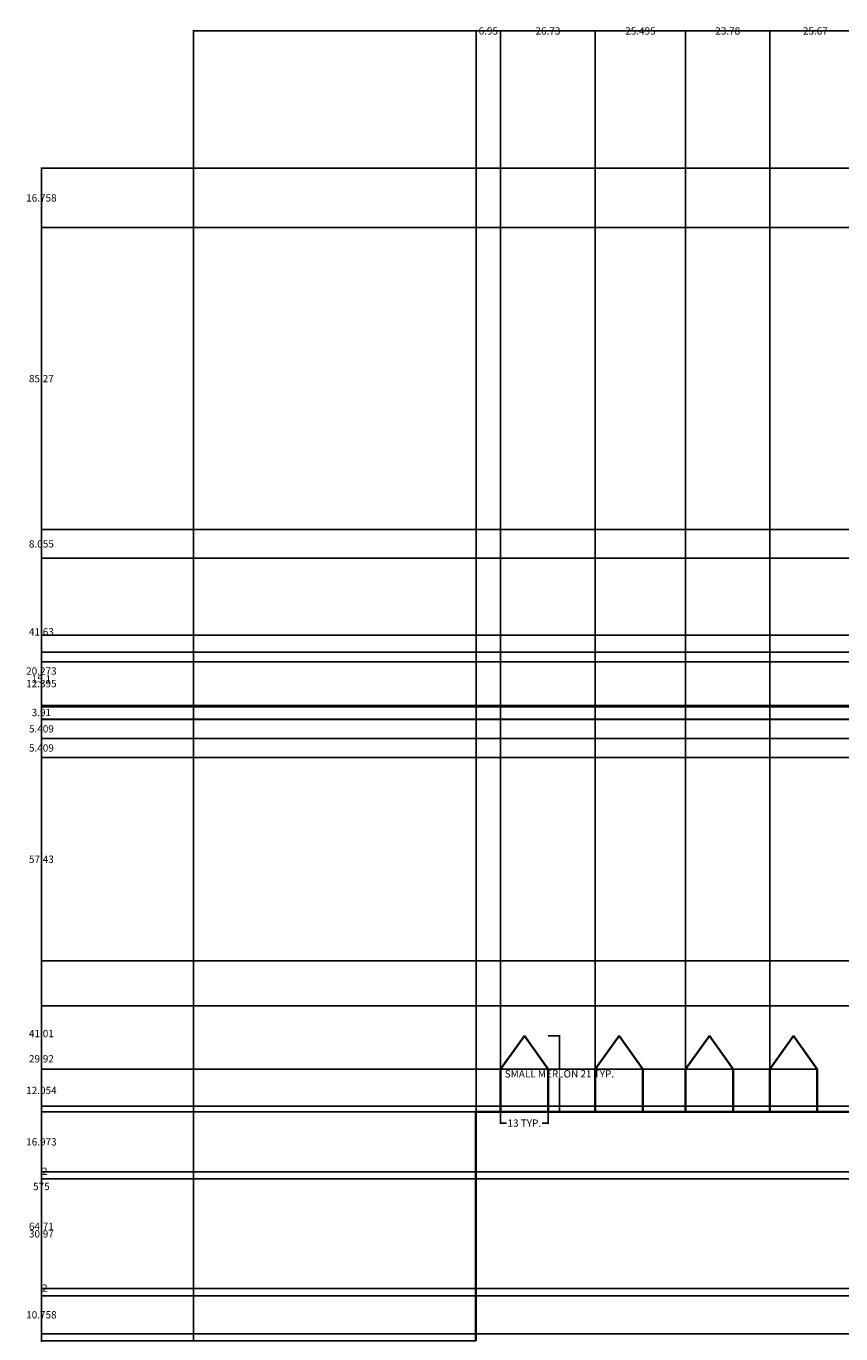
# Model space of a CAD drawing. Units: inches. Extents: x 14 to 859, y 52 to 711.
# Tile 4 of 11: x 14 to 244, y 342 to 711. Entities that reach past the tile are written whole.
import ezdxf

# ---------------------------------------------------------------- set-up
doc = ezdxf.new("R2010")
doc.units = ezdxf.units.IN
doc.header["$MEASUREMENT"] = 0
doc.layers.add('A-ANNO-DIMS', color=2, linetype='Continuous', lineweight=18)
doc.layers.add('A-ELEV', color=7, linetype='Continuous', lineweight=35)
doc.styles.get("Standard").update_dxf_attribs({"font": 'arial.ttf'})
doc.dimstyles.get("Standard").update_dxf_attribs({"dimtxt": 2.0625, "dimasz": 0.18, "dimexe": 0.18, "dimexo": 0.0625, "dimgap": 0.09, "dimtad": 0, "dimtih": 1, "dimtoh": 1, "dimdec": 4, "dimzin": 0, "dimdsep": 46, "dimlunit": 4, "dimtxsty": 'Standard', "dimcen": 0.09, "dimadec": 0, "dimazin": 0, "dimtfac": 1, "dimtdec": 4, "dimtofl": 0, "dimtmove": 0, "dimatfit": 3, "dimfxl": 1, "dimtolj": 1, "dimtzin": 0, "dimarcsym": 0})

# ---------------------------------------------------------------- blocks, each defined once
blk = doc.blocks.new('MERLON-SMALL')
for p, q in [((0, 12.05), (6.7, 21.41)), ((6.7, 21.41), (13.39, 12.05)), ((0, 0), (0, 12.05)), ((13.39, 0), (13.39, 12.05))]:
    blk.add_line(p, q)
blk = doc.blocks.new('*D7')
at = {"layer": 'A-ANNO-DIMS', "color": 0, "lineweight": -2, "transparency": 16777216}
for p, q in [((160.97, 425.79), (164.3, 425.79)), ((164.12, 425.61), (164.12, 416.24)), ((164.12, 404.55), (164.12, 413.92)), ((160.97, 404.37), (164.3, 404.37))]:
    blk.add_line(p, q, dxfattribs=at)
at = {"layer": 'A-ANNO-DIMS', "color": 0, "transparency": 16777216}
for points in [[(164.09, 425.61), (164.15, 425.61), (164.12, 425.79)], [(164.09, 404.55), (164.15, 404.55), (164.12, 404.37)]]:
    blk.add_solid(points, dxfattribs=at)
at = {"layer": 'Defpoints', "color": 0, "transparency": 16777216}
for p in [(160.91, 425.79), (164.12, 425.79), (160.91, 404.37)]:
    blk.add_point(p, dxfattribs=at)
at = {"layer": 'A-ANNO-DIMS', "color": 0, "transparency": 16777216, "insert": (164.12, 415.08), "char_height": 2.0625, "attachment_point": 5}
blk.add_mtext('\\A1;SMALL MERLON 21 TYP.', dxfattribs=at)
blk = doc.blocks.new('*D8')
at = {"layer": 'A-ANNO-DIMS', "color": 0, "lineweight": -2, "transparency": 16777216}
for p, q in [((147.52, 404.31), (147.52, 400.98)), ((160.91, 404.31), (160.91, 400.98)), ((147.7, 401.16), (149.2, 401.16)), ((160.73, 401.16), (159.23, 401.16))]:
    blk.add_line(p, q, dxfattribs=at)
at = {"layer": 'A-ANNO-DIMS', "color": 0, "transparency": 16777216}
for points in [[(147.7, 401.19), (147.7, 401.13), (147.52, 401.16)], [(160.73, 401.19), (160.73, 401.13), (160.91, 401.16)]]:
    blk.add_solid(points, dxfattribs=at)
at = {"layer": 'Defpoints', "color": 0, "transparency": 16777216}
for p in [(147.52, 404.37), (160.91, 404.37), (160.91, 401.16)]:
    blk.add_point(p, dxfattribs=at)
at = {"layer": 'A-ANNO-DIMS', "color": 0, "transparency": 16777216, "insert": (154.21, 401.16), "char_height": 2.0625, "attachment_point": 5}
blk.add_mtext('\\A1;13 TYP.', dxfattribs=at)
blk = doc.blocks.new('*D13')
at = {"layer": 'A-ANNO-DIMS', "color": 0, "lineweight": -2, "transparency": 16777216}
for p, q in [((60.78, 339.73), (60.78, 709.71)), ((60.96, 709.53), (432.6, 709.53)), ((811.37, 709.53), (439.73, 709.53)), ((811.55, 339.73), (811.55, 709.71))]:
    blk.add_line(p, q, dxfattribs=at)
at = {"layer": 'A-ANNO-DIMS', "color": 0, "transparency": 16777216}
for points in [[(60.96, 709.56), (60.96, 709.5), (60.78, 709.53)], [(811.37, 709.56), (811.37, 709.5), (811.55, 709.53)]]:
    blk.add_solid(points, dxfattribs=at)
at = {"layer": 'Defpoints', "color": 0, "transparency": 16777216}
for p in [(811.55, 709.53), (60.78, 339.66), (811.55, 339.66)]:
    blk.add_point(p, dxfattribs=at)
at = {"layer": 'A-ANNO-DIMS', "color": 0, "transparency": 16777216, "insert": (436.17, 709.53), "char_height": 2.062, "attachment_point": 5}
blk.add_mtext('\\A1;750.8', dxfattribs=at)
blk = doc.blocks.new('*D16')
at = {"layer": 'A-ANNO-DIMS', "color": 0, "lineweight": -2, "transparency": 16777216}
for p, q in [((429.96, 670.76), (17.7, 670.76)), ((17.88, 670.58), (17.88, 384.41)), ((17.88, 95.97), (17.88, 382.14)), ((60.72, 95.79), (17.7, 95.79))]:
    blk.add_line(p, q, dxfattribs=at)
at = {"layer": 'A-ANNO-DIMS', "color": 0, "transparency": 16777216}
for points in [[(17.85, 670.58), (17.91, 670.58), (17.88, 670.76)], [(17.85, 95.97), (17.91, 95.97), (17.88, 95.79)]]:
    blk.add_solid(points, dxfattribs=at)
at = {"layer": 'Defpoints', "color": 0, "transparency": 16777216}
for p in [(17.88, 670.76), (430.02, 670.76), (60.78, 95.79)]:
    blk.add_point(p, dxfattribs=at)
at = {"layer": 'A-ANNO-DIMS', "color": 0, "transparency": 16777216, "insert": (17.88, 383.28), "char_height": 2.062, "attachment_point": 5}
blk.add_mtext('\\A1;575', dxfattribs=at)
blk = doc.blocks.new('*D25')
at = {"layer": 'A-ANNO-DIMS', "color": 0, "lineweight": -2, "transparency": 16777216}
for p, q in [((298.67, 341.67), (17.7, 341.67)), ((17.88, 341.49), (17.88, 305.98)), ((17.88, 268.19), (17.88, 303.7)), ((298.67, 268.01), (17.7, 268.01))]:
    blk.add_line(p, q, dxfattribs=at)
at = {"layer": 'A-ANNO-DIMS', "color": 0, "transparency": 16777216}
for points in [[(17.85, 341.49), (17.91, 341.49), (17.88, 341.67)], [(17.85, 268.19), (17.91, 268.19), (17.88, 268.01)]]:
    blk.add_solid(points, dxfattribs=at)
at = {"layer": 'Defpoints', "color": 0, "transparency": 16777216}
for p in [(17.88, 341.67), (298.73, 341.67), (298.73, 268.01)]:
    blk.add_point(p, dxfattribs=at)
at = {"layer": 'A-ANNO-DIMS', "color": 0, "transparency": 16777216, "insert": (17.88, 304.84), "char_height": 2.062, "attachment_point": 5}
blk.add_mtext('\\A1;73.66', dxfattribs=at)
blk = doc.blocks.new('*D26')
at = {"layer": 'A-ANNO-DIMS', "color": 0, "lineweight": -2, "transparency": 16777216}
for p, q in [((287.83, 352.43), (17.7, 352.43)), ((17.88, 352.25), (17.88, 348.19)), ((17.88, 341.85), (17.88, 345.91)), ((298.67, 341.67), (17.7, 341.67))]:
    blk.add_line(p, q, dxfattribs=at)
at = {"layer": 'A-ANNO-DIMS', "color": 0, "transparency": 16777216}
for points in [[(17.85, 352.25), (17.91, 352.25), (17.88, 352.43)], [(17.85, 341.85), (17.91, 341.85), (17.88, 341.67)]]:
    blk.add_solid(points, dxfattribs=at)
at = {"layer": 'Defpoints', "color": 0, "transparency": 16777216}
for p in [(17.88, 352.43), (287.89, 352.43), (298.73, 341.67)]:
    blk.add_point(p, dxfattribs=at)
at = {"layer": 'A-ANNO-DIMS', "color": 0, "transparency": 16777216, "insert": (17.88, 347.05), "char_height": 2.062, "attachment_point": 5}
blk.add_mtext('\\A1;10.758', dxfattribs=at)
blk = doc.blocks.new('*D27')
at = {"layer": 'A-ANNO-DIMS', "color": 0, "lineweight": -2, "transparency": 16777216}
for p, q in [((17.88, 354.43), (17.88, 354.61)), ((17.88, 354.61), (18.06, 354.61)), ((287.83, 354.43), (17.7, 354.43)), ((287.83, 352.43), (17.7, 352.43)), ((17.88, 352.61), (17.88, 354.25))]:
    blk.add_line(p, q, dxfattribs=at)
at = {"layer": 'A-ANNO-DIMS', "color": 0, "transparency": 16777216}
for points in [[(17.85, 354.25), (17.91, 354.25), (17.88, 354.43)], [(17.85, 352.61), (17.91, 352.61), (17.88, 352.43)]]:
    blk.add_solid(points, dxfattribs=at)
at = {"layer": 'Defpoints', "color": 0, "transparency": 16777216}
for p in [(17.88, 354.43), (287.89, 354.43), (287.89, 352.43)]:
    blk.add_point(p, dxfattribs=at)
at = {"layer": 'A-ANNO-DIMS', "color": 0, "transparency": 16777216, "insert": (18.83, 354.61), "char_height": 2.062, "attachment_point": 5}
blk.add_mtext('\\A1;2', dxfattribs=at)
blk = doc.blocks.new('*D28')
at = {"layer": 'A-ANNO-DIMS', "color": 0, "lineweight": -2, "transparency": 16777216}
for p, q in [((289.61, 385.4), (17.7, 385.4)), ((17.88, 385.22), (17.88, 371.06)), ((17.88, 354.61), (17.88, 368.77)), ((287.83, 354.43), (17.7, 354.43))]:
    blk.add_line(p, q, dxfattribs=at)
at = {"layer": 'A-ANNO-DIMS', "color": 0, "transparency": 16777216}
for points in [[(17.85, 385.22), (17.91, 385.22), (17.88, 385.4)], [(17.85, 354.61), (17.91, 354.61), (17.88, 354.43)]]:
    blk.add_solid(points, dxfattribs=at)
at = {"layer": 'Defpoints', "color": 0, "transparency": 16777216}
for p in [(17.88, 385.4), (289.67, 385.4), (287.89, 354.43)]:
    blk.add_point(p, dxfattribs=at)
at = {"layer": 'A-ANNO-DIMS', "color": 0, "transparency": 16777216, "insert": (17.88, 369.91), "char_height": 2.062, "attachment_point": 5}
blk.add_mtext('\\A1;30.97', dxfattribs=at)
blk = doc.blocks.new('*D29')
at = {"layer": 'A-ANNO-DIMS', "color": 0, "lineweight": -2, "transparency": 16777216}
for p, q in [((289.61, 387.4), (17.7, 387.4)), ((289.61, 385.4), (17.7, 385.4)), ((17.88, 387.4), (17.88, 387.58)), ((17.88, 387.58), (18.06, 387.58)), ((17.88, 385.58), (17.88, 387.22))]:
    blk.add_line(p, q, dxfattribs=at)
at = {"layer": 'A-ANNO-DIMS', "color": 0, "transparency": 16777216}
for points in [[(17.85, 387.22), (17.91, 387.22), (17.88, 387.4)], [(17.85, 385.58), (17.91, 385.58), (17.88, 385.4)]]:
    blk.add_solid(points, dxfattribs=at)
at = {"layer": 'Defpoints', "color": 0, "transparency": 16777216}
for p in [(17.88, 387.4), (289.67, 387.4), (289.67, 385.4)]:
    blk.add_point(p, dxfattribs=at)
at = {"layer": 'A-ANNO-DIMS', "color": 0, "transparency": 16777216, "insert": (18.83, 387.58), "char_height": 2.062, "attachment_point": 5}
blk.add_mtext('\\A1;2', dxfattribs=at)
blk = doc.blocks.new('*D30')
at = {"layer": 'A-ANNO-DIMS', "color": 0, "lineweight": -2, "transparency": 16777216}
for p, q in [((287.83, 404.37), (17.7, 404.37)), ((17.88, 404.19), (17.88, 397.03)), ((17.88, 387.58), (17.88, 394.74)), ((289.61, 387.4), (17.7, 387.4))]:
    blk.add_line(p, q, dxfattribs=at)
at = {"layer": 'A-ANNO-DIMS', "color": 0, "transparency": 16777216}
for points in [[(17.85, 404.19), (17.91, 404.19), (17.88, 404.37)], [(17.85, 387.58), (17.91, 387.58), (17.88, 387.4)]]:
    blk.add_solid(points, dxfattribs=at)
at = {"layer": 'Defpoints', "color": 0, "transparency": 16777216}
for p in [(17.88, 404.37), (287.89, 404.37), (289.67, 387.4)]:
    blk.add_point(p, dxfattribs=at)
at = {"layer": 'A-ANNO-DIMS', "color": 0, "transparency": 16777216, "insert": (17.88, 395.88), "char_height": 2.062, "attachment_point": 5}
blk.add_mtext('\\A1;16.973', dxfattribs=at)
blk = doc.blocks.new('*D59')
at = {"layer": 'A-ANNO-DIMS', "color": 0, "lineweight": -2, "transparency": 16777216}
for p, q in [((140.51, 404.37), (17.7, 404.37)), ((17.88, 404.19), (17.88, 373.16)), ((17.88, 339.84), (17.88, 370.87)), ((140.51, 339.66), (17.7, 339.66))]:
    blk.add_line(p, q, dxfattribs=at)
at = {"layer": 'A-ANNO-DIMS', "color": 0, "transparency": 16777216}
for points in [[(17.85, 404.19), (17.91, 404.19), (17.88, 404.37)], [(17.85, 339.84), (17.91, 339.84), (17.88, 339.66)]]:
    blk.add_solid(points, dxfattribs=at)
at = {"layer": 'Defpoints', "color": 0, "transparency": 16777216}
for p in [(17.88, 404.37), (140.57, 404.37), (140.57, 339.66)]:
    blk.add_point(p, dxfattribs=at)
at = {"layer": 'A-ANNO-DIMS', "color": 0, "transparency": 16777216, "insert": (17.88, 372.02), "char_height": 2.062, "attachment_point": 5}
blk.add_mtext('\\A1;64.71', dxfattribs=at)
blk = doc.blocks.new('*D60')
at = {"layer": 'A-ANNO-DIMS', "color": 0, "lineweight": -2, "transparency": 16777216}
for p, q in [((236.85, 416.42), (17.7, 416.42)), ((17.88, 416.24), (17.88, 411.54)), ((17.88, 404.55), (17.88, 409.25)), ((236.85, 404.37), (17.7, 404.37))]:
    blk.add_line(p, q, dxfattribs=at)
at = {"layer": 'A-ANNO-DIMS', "color": 0, "transparency": 16777216}
for points in [[(17.85, 416.24), (17.91, 416.24), (17.88, 416.42)], [(17.85, 404.55), (17.91, 404.55), (17.88, 404.37)]]:
    blk.add_solid(points, dxfattribs=at)
at = {"layer": 'Defpoints', "color": 0, "transparency": 16777216}
for p in [(17.88, 416.42), (236.92, 416.42), (236.92, 404.37)]:
    blk.add_point(p, dxfattribs=at)
at = {"layer": 'A-ANNO-DIMS', "color": 0, "transparency": 16777216, "insert": (17.88, 410.4), "char_height": 2.062, "attachment_point": 5}
blk.add_mtext('\\A1;12.054', dxfattribs=at)
blk = doc.blocks.new('*D62')
at = {"layer": 'A-ANNO-DIMS', "color": 0, "lineweight": -2, "transparency": 16777216}
for p, q in [((140.57, 404.43), (140.57, 709.71)), ((140.75, 709.53), (141.26, 709.53)), ((147.34, 709.53), (146.83, 709.53)), ((147.52, 404.43), (147.52, 709.71))]:
    blk.add_line(p, q, dxfattribs=at)
at = {"layer": 'A-ANNO-DIMS', "color": 0, "transparency": 16777216}
for points in [[(140.75, 709.56), (140.75, 709.5), (140.57, 709.53)], [(147.34, 709.56), (147.34, 709.5), (147.52, 709.53)]]:
    blk.add_solid(points, dxfattribs=at)
at = {"layer": 'Defpoints', "color": 0, "transparency": 16777216}
for p in [(147.52, 709.53), (140.57, 404.37), (147.52, 404.37)]:
    blk.add_point(p, dxfattribs=at)
at = {"layer": 'A-ANNO-DIMS', "color": 0, "transparency": 16777216, "insert": (144.04, 709.53), "char_height": 2.062, "attachment_point": 5}
blk.add_mtext('\\A1;6.95', dxfattribs=at)
blk = doc.blocks.new('*D63')
at = {"layer": 'A-ANNO-DIMS', "color": 0, "lineweight": -2, "transparency": 16777216}
for p, q in [((147.52, 404.43), (147.52, 709.71)), ((147.7, 709.53), (157.3, 709.53)), ((174.07, 709.53), (164.47, 709.53)), ((174.25, 404.43), (174.25, 709.71))]:
    blk.add_line(p, q, dxfattribs=at)
at = {"layer": 'A-ANNO-DIMS', "color": 0, "transparency": 16777216}
for points in [[(147.7, 709.56), (147.7, 709.5), (147.52, 709.53)], [(174.07, 709.56), (174.07, 709.5), (174.25, 709.53)]]:
    blk.add_solid(points, dxfattribs=at)
at = {"layer": 'Defpoints', "color": 0, "transparency": 16777216}
for p in [(174.25, 709.53), (147.52, 404.37), (174.25, 404.37)]:
    blk.add_point(p, dxfattribs=at)
at = {"layer": 'A-ANNO-DIMS', "color": 0, "transparency": 16777216, "insert": (160.88, 709.53), "char_height": 2.062, "attachment_point": 5}
blk.add_mtext('\\A1;26.73', dxfattribs=at)
blk = doc.blocks.new('*D64')
at = {"layer": 'A-ANNO-DIMS', "color": 0, "lineweight": -2, "transparency": 16777216}
for p, q in [((174.25, 404.43), (174.25, 709.71)), ((174.43, 709.53), (182.6, 709.53)), ((199.56, 709.53), (191.39, 709.53)), ((199.74, 404.43), (199.74, 709.71))]:
    blk.add_line(p, q, dxfattribs=at)
at = {"layer": 'A-ANNO-DIMS', "color": 0, "transparency": 16777216}
for points in [[(174.43, 709.56), (174.43, 709.5), (174.25, 709.53)], [(199.56, 709.56), (199.56, 709.5), (199.74, 709.53)]]:
    blk.add_solid(points, dxfattribs=at)
at = {"layer": 'Defpoints', "color": 0, "transparency": 16777216}
for p in [(199.74, 709.53), (174.25, 404.37), (199.74, 404.37)]:
    blk.add_point(p, dxfattribs=at)
at = {"layer": 'A-ANNO-DIMS', "color": 0, "transparency": 16777216, "insert": (187, 709.53), "char_height": 2.062, "attachment_point": 5}
blk.add_mtext('\\A1;25.495', dxfattribs=at)
blk = doc.blocks.new('*D65')
at = {"layer": 'A-ANNO-DIMS', "color": 0, "lineweight": -2, "transparency": 16777216}
for p, q in [((199.74, 404.43), (199.74, 709.71)), ((199.92, 709.53), (208.05, 709.53)), ((223.35, 709.53), (215.22, 709.53)), ((223.53, 404.43), (223.53, 709.71))]:
    blk.add_line(p, q, dxfattribs=at)
at = {"layer": 'A-ANNO-DIMS', "color": 0, "transparency": 16777216}
for points in [[(199.92, 709.56), (199.92, 709.5), (199.74, 709.53)], [(223.35, 709.56), (223.35, 709.5), (223.53, 709.53)]]:
    blk.add_solid(points, dxfattribs=at)
at = {"layer": 'Defpoints', "color": 0, "transparency": 16777216}
for p in [(223.53, 709.53), (199.74, 404.37), (223.53, 404.37)]:
    blk.add_point(p, dxfattribs=at)
at = {"layer": 'A-ANNO-DIMS', "color": 0, "transparency": 16777216, "insert": (211.63, 709.53), "char_height": 2.062, "attachment_point": 5}
blk.add_mtext('\\A1;23.78', dxfattribs=at)
blk = doc.blocks.new('*D66')
at = {"layer": 'A-ANNO-DIMS', "color": 0, "lineweight": -2, "transparency": 16777216}
for p, q in [((223.53, 404.43), (223.53, 709.71)), ((223.71, 709.53), (232.77, 709.53)), ((249.01, 709.53), (239.95, 709.53)), ((249.19, 404.43), (249.19, 709.71))]:
    blk.add_line(p, q, dxfattribs=at)
at = {"layer": 'A-ANNO-DIMS', "color": 0, "transparency": 16777216}
for points in [[(223.71, 709.56), (223.71, 709.5), (223.53, 709.53)], [(249.01, 709.56), (249.01, 709.5), (249.19, 709.53)]]:
    blk.add_solid(points, dxfattribs=at)
at = {"layer": 'Defpoints', "color": 0, "transparency": 16777216}
for p in [(249.19, 709.53), (223.53, 404.37), (249.19, 404.37)]:
    blk.add_point(p, dxfattribs=at)
at = {"layer": 'A-ANNO-DIMS', "color": 0, "transparency": 16777216, "insert": (236.36, 709.53), "char_height": 2.062, "attachment_point": 5}
blk.add_mtext('\\A1;25.67', dxfattribs=at)
blk = doc.blocks.new('*D86')
at = {"layer": 'A-ANNO-DIMS', "color": 0, "lineweight": -2, "transparency": 16777216}
for p, q in [((366.44, 446.95), (17.7, 446.95)), ((17.88, 446.77), (17.88, 427.59)), ((17.88, 406.12), (17.88, 425.3)), ((276.44, 405.94), (17.7, 405.94))]:
    blk.add_line(p, q, dxfattribs=at)
at = {"layer": 'A-ANNO-DIMS', "color": 0, "transparency": 16777216}
for points in [[(17.85, 446.77), (17.91, 446.77), (17.88, 446.95)], [(17.85, 406.12), (17.91, 406.12), (17.88, 405.94)]]:
    blk.add_solid(points, dxfattribs=at)
at = {"layer": 'Defpoints', "color": 0, "transparency": 16777216}
for p in [(17.88, 446.95), (366.51, 446.95), (276.5, 405.94)]:
    blk.add_point(p, dxfattribs=at)
at = {"layer": 'A-ANNO-DIMS', "color": 0, "transparency": 16777216, "insert": (17.88, 426.45), "char_height": 2.062, "attachment_point": 5}
blk.add_mtext('\\A1;41.01', dxfattribs=at)
blk = doc.blocks.new('*D87')
at = {"layer": 'A-ANNO-DIMS', "color": 0, "lineweight": -2, "transparency": 16777216}
for p, q in [((276.44, 504.38), (17.7, 504.38)), ((17.88, 504.2), (17.88, 476.81)), ((17.88, 447.13), (17.88, 474.52)), ((366.44, 446.95), (17.7, 446.95))]:
    blk.add_line(p, q, dxfattribs=at)
at = {"layer": 'A-ANNO-DIMS', "color": 0, "transparency": 16777216}
for points in [[(17.85, 504.2), (17.91, 504.2), (17.88, 504.38)], [(17.85, 447.13), (17.91, 447.13), (17.88, 446.95)]]:
    blk.add_solid(points, dxfattribs=at)
at = {"layer": 'Defpoints', "color": 0, "transparency": 16777216}
for p in [(17.88, 504.38), (276.5, 504.38), (366.51, 446.95)]:
    blk.add_point(p, dxfattribs=at)
at = {"layer": 'A-ANNO-DIMS', "color": 0, "transparency": 16777216, "insert": (17.88, 475.67), "char_height": 2.062, "attachment_point": 5}
blk.add_mtext('\\A1;57.43', dxfattribs=at)
blk = doc.blocks.new('*D88')
at = {"layer": 'A-ANNO-DIMS', "color": 0, "lineweight": -2, "transparency": 16777216}
for p, q in [((276.44, 509.79), (17.7, 509.79)), ((17.88, 509.61), (17.88, 508.23)), ((17.88, 504.56), (17.88, 505.94)), ((276.44, 504.38), (17.7, 504.38))]:
    blk.add_line(p, q, dxfattribs=at)
at = {"layer": 'A-ANNO-DIMS', "color": 0, "transparency": 16777216}
for points in [[(17.85, 509.61), (17.91, 509.61), (17.88, 509.79)], [(17.85, 504.56), (17.91, 504.56), (17.88, 504.38)]]:
    blk.add_solid(points, dxfattribs=at)
at = {"layer": 'Defpoints', "color": 0, "transparency": 16777216}
for p in [(17.88, 509.79), (276.5, 509.79), (276.5, 504.38)]:
    blk.add_point(p, dxfattribs=at)
at = {"layer": 'A-ANNO-DIMS', "color": 0, "transparency": 16777216, "insert": (17.88, 507.09), "char_height": 2.062, "attachment_point": 5}
blk.add_mtext('\\A1;5.409', dxfattribs=at)
blk = doc.blocks.new('*D89')
at = {"layer": 'A-ANNO-DIMS', "color": 0, "lineweight": -2, "transparency": 16777216}
for p, q in [((269.65, 515.2), (17.7, 515.2)), ((17.88, 515.02), (17.88, 513.64)), ((269.65, 509.79), (17.7, 509.79)), ((17.88, 509.97), (17.88, 511.35))]:
    blk.add_line(p, q, dxfattribs=at)
at = {"layer": 'A-ANNO-DIMS', "color": 0, "transparency": 16777216}
for points in [[(17.85, 515.02), (17.91, 515.02), (17.88, 515.2)], [(17.85, 509.97), (17.91, 509.97), (17.88, 509.79)]]:
    blk.add_solid(points, dxfattribs=at)
at = {"layer": 'Defpoints', "color": 0, "transparency": 16777216}
for p in [(17.88, 515.2), (269.71, 515.2), (269.71, 509.79)]:
    blk.add_point(p, dxfattribs=at)
at = {"layer": 'A-ANNO-DIMS', "color": 0, "transparency": 16777216, "insert": (17.88, 512.49), "char_height": 2.062, "attachment_point": 5}
blk.add_mtext('\\A1;5.409', dxfattribs=at)
blk = doc.blocks.new('*D90')
at = {"layer": 'A-ANNO-DIMS', "color": 0, "lineweight": -2, "transparency": 16777216}
for p, q in [((264.56, 519.05), (17.7, 519.05)), ((17.88, 518.87), (17.88, 518.24)), ((264.56, 515.14), (17.7, 515.14)), ((17.88, 515.32), (17.88, 515.95))]:
    blk.add_line(p, q, dxfattribs=at)
at = {"layer": 'A-ANNO-DIMS', "color": 0, "transparency": 16777216}
for points in [[(17.85, 518.87), (17.91, 518.87), (17.88, 519.05)], [(17.85, 515.32), (17.91, 515.32), (17.88, 515.14)]]:
    blk.add_solid(points, dxfattribs=at)
at = {"layer": 'Defpoints', "color": 0, "transparency": 16777216}
for p in [(17.88, 519.05), (264.63, 519.05), (264.63, 515.14)]:
    blk.add_point(p, dxfattribs=at)
at = {"layer": 'A-ANNO-DIMS', "color": 0, "transparency": 16777216, "insert": (17.88, 517.1), "char_height": 2.062, "attachment_point": 5}
blk.add_mtext('\\A1;3.91', dxfattribs=at)
blk = doc.blocks.new('*D91')
at = {"layer": 'A-ANNO-DIMS', "color": 0, "lineweight": -2, "transparency": 16777216}
for p, q in [((306.8, 560.68), (17.7, 560.68)), ((17.88, 560.5), (17.88, 541.01)), ((17.88, 519.23), (17.88, 538.72)), ((264.56, 519.05), (17.7, 519.05))]:
    blk.add_line(p, q, dxfattribs=at)
at = {"layer": 'A-ANNO-DIMS', "color": 0, "transparency": 16777216}
for points in [[(17.85, 560.5), (17.91, 560.5), (17.88, 560.68)], [(17.85, 519.23), (17.91, 519.23), (17.88, 519.05)]]:
    blk.add_solid(points, dxfattribs=at)
at = {"layer": 'Defpoints', "color": 0, "transparency": 16777216}
for p in [(17.88, 560.68), (306.86, 560.68), (264.63, 519.05)]:
    blk.add_point(p, dxfattribs=at)
at = {"layer": 'A-ANNO-DIMS', "color": 0, "transparency": 16777216, "insert": (17.88, 539.87), "char_height": 2.062, "attachment_point": 5}
blk.add_mtext('\\A1;41.63', dxfattribs=at)
blk = doc.blocks.new('*D92')
at = {"layer": 'A-ANNO-DIMS', "color": 0, "lineweight": -2, "transparency": 16777216}
for p, q in [((342.81, 568.74), (17.7, 568.74)), ((17.88, 568.56), (17.88, 565.85)), ((17.88, 560.86), (17.88, 563.57)), ((306.8, 560.68), (17.7, 560.68))]:
    blk.add_line(p, q, dxfattribs=at)
at = {"layer": 'A-ANNO-DIMS', "color": 0, "transparency": 16777216}
for points in [[(17.85, 568.56), (17.91, 568.56), (17.88, 568.74)], [(17.85, 560.86), (17.91, 560.86), (17.88, 560.68)]]:
    blk.add_solid(points, dxfattribs=at)
at = {"layer": 'Defpoints', "color": 0, "transparency": 16777216}
for p in [(17.88, 568.74), (342.87, 568.74), (306.86, 560.68)]:
    blk.add_point(p, dxfattribs=at)
at = {"layer": 'A-ANNO-DIMS', "color": 0, "transparency": 16777216, "insert": (17.88, 564.71), "char_height": 2.062, "attachment_point": 5}
blk.add_mtext('\\A1;8.055', dxfattribs=at)
blk = doc.blocks.new('*D93')
at = {"layer": 'A-ANNO-DIMS', "color": 0, "lineweight": -2, "transparency": 16777216}
for p, q in [((429.22, 654.01), (17.7, 654.01)), ((17.88, 653.83), (17.88, 612.51)), ((17.88, 568.92), (17.88, 610.23)), ((342.81, 568.74), (17.7, 568.74))]:
    blk.add_line(p, q, dxfattribs=at)
at = {"layer": 'A-ANNO-DIMS', "color": 0, "transparency": 16777216}
for points in [[(17.85, 653.83), (17.91, 653.83), (17.88, 654.01)], [(17.85, 568.92), (17.91, 568.92), (17.88, 568.74)]]:
    blk.add_solid(points, dxfattribs=at)
at = {"layer": 'Defpoints', "color": 0, "transparency": 16777216}
for p in [(17.88, 654.01), (429.29, 654.01), (342.87, 568.74)]:
    blk.add_point(p, dxfattribs=at)
at = {"layer": 'A-ANNO-DIMS', "color": 0, "transparency": 16777216, "insert": (17.88, 611.37), "char_height": 2.062, "attachment_point": 5}
blk.add_mtext('\\A1;85.27', dxfattribs=at)
blk = doc.blocks.new('*D94')
at = {"layer": 'A-ANNO-DIMS', "color": 0, "lineweight": -2, "transparency": 16777216}
for p, q in [((429.96, 670.76), (17.7, 670.76)), ((17.88, 670.58), (17.88, 663.53)), ((17.88, 654.19), (17.88, 661.24)), ((429.22, 654.01), (17.7, 654.01))]:
    blk.add_line(p, q, dxfattribs=at)
at = {"layer": 'A-ANNO-DIMS', "color": 0, "transparency": 16777216}
for points in [[(17.85, 670.58), (17.91, 670.58), (17.88, 670.76)], [(17.85, 654.19), (17.91, 654.19), (17.88, 654.01)]]:
    blk.add_solid(points, dxfattribs=at)
at = {"layer": 'Defpoints', "color": 0, "transparency": 16777216}
for p in [(17.88, 670.76), (430.02, 670.76), (429.29, 654.01)]:
    blk.add_point(p, dxfattribs=at)
at = {"layer": 'A-ANNO-DIMS', "color": 0, "transparency": 16777216, "insert": (17.88, 662.38), "char_height": 2.062, "attachment_point": 5}
blk.add_mtext('\\A1;16.758', dxfattribs=at)
blk = doc.blocks.new('*D113')
at = {"layer": 'A-ANNO-DIMS', "color": 0, "lineweight": -2, "transparency": 16777216}
for p, q in [((344.62, 538.94), (17.7, 538.94)), ((17.88, 538.76), (17.88, 529.95)), ((17.88, 518.85), (17.88, 527.66)), ((306.8, 518.67), (17.7, 518.67))]:
    blk.add_line(p, q, dxfattribs=at)
at = {"layer": 'A-ANNO-DIMS', "color": 0, "transparency": 16777216}
for points in [[(17.85, 538.76), (17.91, 538.76), (17.88, 538.94)], [(17.85, 518.85), (17.91, 518.85), (17.88, 518.67)]]:
    blk.add_solid(points, dxfattribs=at)
at = {"layer": 'Defpoints', "color": 0, "transparency": 16777216}
for p in [(17.88, 538.94), (344.68, 538.94), (306.86, 518.67)]:
    blk.add_point(p, dxfattribs=at)
at = {"layer": 'A-ANNO-DIMS', "color": 0, "transparency": 16777216, "insert": (17.88, 528.81), "char_height": 2.062, "attachment_point": 5}
blk.add_mtext('\\A1;20.273', dxfattribs=at)
blk = doc.blocks.new('*D116')
at = {"layer": 'A-ANNO-DIMS', "color": 0, "lineweight": -2, "transparency": 16777216}
for p, q in [((435.99, 534.15), (17.7, 534.15)), ((17.88, 533.97), (17.88, 527.74)), ((17.88, 519.23), (17.88, 525.46)), ((435.99, 519.05), (17.7, 519.05))]:
    blk.add_line(p, q, dxfattribs=at)
at = {"layer": 'A-ANNO-DIMS', "color": 0, "transparency": 16777216}
for points in [[(17.85, 533.97), (17.91, 533.97), (17.88, 534.15)], [(17.85, 519.23), (17.91, 519.23), (17.88, 519.05)]]:
    blk.add_solid(points, dxfattribs=at)
at = {"layer": 'Defpoints', "color": 0, "transparency": 16777216}
for p in [(17.88, 534.15), (436.05, 534.15), (436.05, 519.05)]:
    blk.add_point(p, dxfattribs=at)
at = {"layer": 'A-ANNO-DIMS', "color": 0, "transparency": 16777216, "insert": (17.88, 526.6), "char_height": 2.062, "attachment_point": 5}
blk.add_mtext('\\A1;15.1', dxfattribs=at)
blk = doc.blocks.new('*D117')
at = {"layer": 'A-ANNO-DIMS', "color": 0, "lineweight": -2, "transparency": 16777216}
for p, q in [((433.29, 531.45), (17.7, 531.45)), ((17.88, 531.27), (17.88, 526.39)), ((17.88, 519.23), (17.88, 524.11)), ((433.29, 519.05), (17.7, 519.05))]:
    blk.add_line(p, q, dxfattribs=at)
at = {"layer": 'A-ANNO-DIMS', "color": 0, "transparency": 16777216}
for points in [[(17.85, 531.27), (17.91, 531.27), (17.88, 531.45)], [(17.85, 519.23), (17.91, 519.23), (17.88, 519.05)]]:
    blk.add_solid(points, dxfattribs=at)
at = {"layer": 'Defpoints', "color": 0, "transparency": 16777216}
for p in [(17.88, 531.45), (433.35, 531.45), (433.35, 519.05)]:
    blk.add_point(p, dxfattribs=at)
at = {"layer": 'A-ANNO-DIMS', "color": 0, "transparency": 16777216, "insert": (17.88, 525.25), "char_height": 2.062, "attachment_point": 5}
blk.add_mtext('\\A1;12.395', dxfattribs=at)
blk = doc.blocks.new('*D124')
at = {"layer": 'A-ANNO-DIMS', "color": 0, "lineweight": -2, "transparency": 16777216}
for p, q in [((324.12, 434.29), (17.7, 434.29)), ((17.88, 434.11), (17.88, 420.48)), ((17.88, 404.55), (17.88, 418.19)), ((324.12, 404.37), (17.7, 404.37))]:
    blk.add_line(p, q, dxfattribs=at)
at = {"layer": 'A-ANNO-DIMS', "color": 0, "transparency": 16777216}
for points in [[(17.85, 434.11), (17.91, 434.11), (17.88, 434.29)], [(17.85, 404.55), (17.91, 404.55), (17.88, 404.37)]]:
    blk.add_solid(points, dxfattribs=at)
at = {"layer": 'Defpoints', "color": 0, "transparency": 16777216}
for p in [(17.88, 434.29), (324.18, 434.29), (324.18, 404.37)]:
    blk.add_point(p, dxfattribs=at)
at = {"layer": 'A-ANNO-DIMS', "color": 0, "transparency": 16777216, "insert": (17.88, 419.33), "char_height": 2.062, "attachment_point": 5}
blk.add_mtext('\\A1;29.92', dxfattribs=at)

msp = doc.modelspace()

# ---------------------------------------------------------------- linework, layer by layer
at = {"layer": 'A-ELEV'}
for p, q in [((140.5683, 339.6626), (140.5683, 404.3712)), ((140.5683, 404.3712), (262.6537, 404.3712))]:
    msp.add_line(p, q, dxfattribs=at)

# ---------------------------------------------------------------- block references
for p in [(147.518, 404.371), (174.2485, 404.371), (199.7436, 404.371), (223.5254, 404.371)]:
    msp.add_blockref('MERLON-SMALL', p, dxfattribs=at)

# ---------------------------------------------------------------- dimensions: what is measured, and where the dimension line sits
at = {"layer": 'A-ANNO-DIMS'}
for base, p1, p2, override, picture, middle in [((811.5534, 709.5262), (60.7804, 339.6626), (811.5534, 339.6626), {"dimdec": 1, "dimlfac": 1, "dimrnd": 0, "dimzin": 0, "dimdsep": 46, "dimlunit": 2}, '*D13', (436.1669, 709.5262)), ((147.5183, 709.5262), (140.5683, 404.3712), (147.5183, 404.3712), {"dimdec": 2, "dimlfac": 1, "dimrnd": 0, "dimzin": 0, "dimdsep": 46, "dimlunit": 2}, '*D62', (144.0433, 709.5262)), ((174.2488, 709.5262), (147.5183, 404.3712), (174.2488, 404.3712), {"dimdec": 2, "dimlfac": 1, "dimrnd": 0, "dimzin": 0, "dimdsep": 46, "dimlunit": 2}, '*D63', (160.8835, 709.5262)), ((199.7439, 709.5262), (174.2488, 404.3712), (199.7439, 404.3712), {"dimdec": 3, "dimlfac": 1, "dimrnd": 0, "dimzin": 0, "dimdsep": 46, "dimlunit": 2}, '*D64', (186.9963, 709.5262)), ((223.5256, 709.5262), (199.7439, 404.3712), (223.5256, 404.3712), {"dimdec": 2, "dimlfac": 1, "dimrnd": 0, "dimzin": 0, "dimdsep": 46, "dimlunit": 2}, '*D65', (211.6348, 709.5262)), ((249.1939, 709.5262), (223.5256, 404.3712), (249.1939, 404.3712), {"dimdec": 2, "dimlfac": 1, "dimrnd": 0, "dimzin": 0, "dimdsep": 46, "dimlunit": 2}, '*D66', (236.3598, 709.5262))]:
    dim = msp.add_linear_dim(base=base, p1=p1, p2=p2, dimstyle='Standard', override=override, dxfattribs=at)
    dim.commit()
    dim.dimension.update_dxf_attribs({"geometry": picture, "text_midpoint": middle})
for base, p1, p2, override, picture, middle in [((17.8785, 670.7637), (429.2862, 654.0061), (430.0228, 670.7637), {"dimdec": 3, "dimlfac": 1, "dimrnd": 0, "dimzin": 0, "dimdsep": 46, "dimlunit": 2}, '*D94', (17.8785, 662.3849)), ((17.8785, 670.7637), (60.7804, 95.7876), (430.0228, 670.7637), {"dimdec": 0, "dimlfac": 1, "dimrnd": 0, "dimzin": 0, "dimdsep": 46, "dimlunit": 2}, '*D16', (17.8785, 383.2756)), ((17.8785, 654.0061), (342.8739, 568.7358), (429.2862, 654.0061), {"dimdec": 2, "dimlfac": 1, "dimrnd": 0, "dimzin": 0, "dimdsep": 46, "dimlunit": 2}, '*D93', (17.8785, 611.371)), ((17.8785, 568.7358), (306.8606, 560.6808), (342.8739, 568.7358), {"dimdec": 3, "dimlfac": 1, "dimrnd": 0, "dimzin": 0, "dimdsep": 46, "dimlunit": 2}, '*D92', (17.8785, 564.7083)), ((17.8785, 560.6808), (264.6274, 519.0512), (306.8606, 560.6808), {"dimdec": 2, "dimlfac": 1, "dimrnd": 0, "dimzin": 0, "dimdsep": 46, "dimlunit": 2}, '*D91', (17.8785, 539.866)), ((17.8785, 538.9419), (306.8606, 518.6693), (344.6778, 538.9419), {"dimdec": 3, "dimlfac": 1, "dimrnd": 0, "dimzin": 0, "dimdsep": 46, "dimlunit": 2}, '*D113', (17.8785, 528.8056)), ((17.8785, 534.1509), (436.0547, 519.0512), (436.0547, 534.1509), {"dimdec": 1, "dimlfac": 1, "dimrnd": 0, "dimzin": 0, "dimdsep": 46, "dimlunit": 2}, '*D116', (17.8785, 526.601)), ((17.8785, 531.4465), (433.3504, 519.0512), (433.3504, 531.4465), {"dimdec": 3, "dimlfac": 1, "dimrnd": 0, "dimzin": 0, "dimdsep": 46, "dimlunit": 2}, '*D117', (17.8785, 525.2488)), ((17.8785, 519.0512), (264.6274, 515.1437), (264.6274, 519.0512), {"dimdec": 2, "dimlfac": 1, "dimrnd": 0, "dimzin": 0, "dimdsep": 46, "dimlunit": 2}, '*D90', (17.8785, 517.0975)), ((17.8785, 515.1991), (269.7112, 509.7903), (269.7112, 515.1991), {"dimdec": 3, "dimlfac": 1, "dimrnd": 0, "dimzin": 0, "dimdsep": 46, "dimlunit": 2}, '*D89', (17.8785, 512.4947)), ((17.8785, 509.7903), (276.5038, 504.3815), (276.5038, 509.7903), {"dimdec": 3, "dimlfac": 1, "dimrnd": 0, "dimzin": 0, "dimdsep": 46, "dimlunit": 2}, '*D88', (17.8785, 507.0859)), ((17.8785, 504.3815), (366.507, 446.9501), (276.5038, 504.3815), {"dimdec": 2, "dimlfac": 1, "dimrnd": 0, "dimzin": 0, "dimdsep": 46, "dimlunit": 2}, '*D87', (17.8785, 475.6658)), ((17.8785, 446.9501), (276.5038, 405.9412), (366.507, 446.9501), {"dimdec": 2, "dimlfac": 1, "dimrnd": 0, "dimzin": 0, "dimdsep": 46, "dimlunit": 2}, '*D86', (17.8785, 426.4456)), ((17.8785, 434.2929), (324.1777, 404.3712), (324.1777, 434.2929), {"dimdec": 2, "dimlfac": 1, "dimrnd": 0, "dimzin": 0, "dimdsep": 46, "dimlunit": 2}, '*D124', (17.8785, 419.332)), ((17.8785, 416.4248), (236.9155, 404.3712), (236.9155, 416.4248), {"dimdec": 3, "dimlfac": 1, "dimrnd": 0, "dimzin": 0, "dimdsep": 46, "dimlunit": 2}, '*D60', (17.8785, 410.398)), ((17.8785, 404.3712), (289.67, 387.3985), (287.893, 404.3712), {"dimdec": 3, "dimlfac": 1, "dimrnd": 0, "dimzin": 0, "dimdsep": 46, "dimlunit": 2}, '*D30', (17.8785, 395.8849)), ((17.8785, 404.3712), (140.5683, 339.6626), (140.5683, 404.3712), {"dimdec": 2, "dimlfac": 1, "dimrnd": 0, "dimzin": 0, "dimdsep": 46, "dimlunit": 2}, '*D59', (17.8785, 372.0169)), ((17.8785, 387.3985), (289.67, 385.3985), (289.67, 387.3985), {"dimdec": 0, "dimlfac": 1, "dimrnd": 0, "dimzin": 0, "dimdsep": 46, "dimlunit": 2}, '*D29', (18.8315, 387.5785)), ((17.8785, 385.3985), (287.893, 354.4291), (289.67, 385.3985), {"dimdec": 2, "dimlfac": 1, "dimrnd": 0, "dimzin": 0, "dimdsep": 46, "dimlunit": 2}, '*D28', (17.8785, 369.9138)), ((17.8785, 354.4291), (287.893, 352.4291), (287.893, 354.4291), {"dimdec": 0, "dimlfac": 1, "dimrnd": 0, "dimzin": 0, "dimdsep": 46, "dimlunit": 2}, '*D27', (18.8315, 354.6091)), ((17.87849, 352.42914), (298.72949, 341.67161), (287.89298, 352.42914), {"dimdec": 3, "dimlfac": 1, "dimrnd": 0, "dimzin": 0, "dimdsep": 46, "dimlunit": 2}, '*D26', (17.87849, 347.05038)), ((17.8785, 341.6716), (298.7295, 268.0097), (298.7295, 341.6716), {"dimdec": 2, "dimlfac": 1, "dimrnd": 0, "dimzin": 0, "dimdsep": 46, "dimlunit": 2}, '*D25', (17.8785, 304.8406))]:
    dim = msp.add_linear_dim(base=base, p1=p1, p2=p2, angle=90, dimstyle='Standard', override=override, dxfattribs=at)
    dim.commit()
    dim.dimension.update_dxf_attribs({"geometry": picture, "text_midpoint": middle})
dim = msp.add_linear_dim(base=(164.1202, 425.7853), p1=(160.9081, 404.3712), p2=(160.9081, 425.7853), angle=90, text='SMALL MERLON <> TYP.', dimstyle='Standard', override={"dimdec": 0, "dimlfac": 1, "dimrnd": 0, "dimzin": 0, "dimdsep": 46, "dimlunit": 2}, dxfattribs=at)
dim.commit()
dim.dimension.update_dxf_attribs({"geometry": '*D7', "text_midpoint": (164.1202, 415.0783)})
dim = msp.add_linear_dim(base=(160.9081, 401.1591), p1=(147.5183, 404.3712), p2=(160.9081, 404.3712), text='<> TYP.', dimstyle='Standard', override={"dimdec": 0, "dimlfac": 1, "dimrnd": 0, "dimzin": 0, "dimdsep": 46, "dimlunit": 2}, dxfattribs=at)
dim.commit()
dim.dimension.update_dxf_attribs({"geometry": '*D8', "text_midpoint": (154.2132, 401.1591)})

doc.saveas('drawing.dxf')
